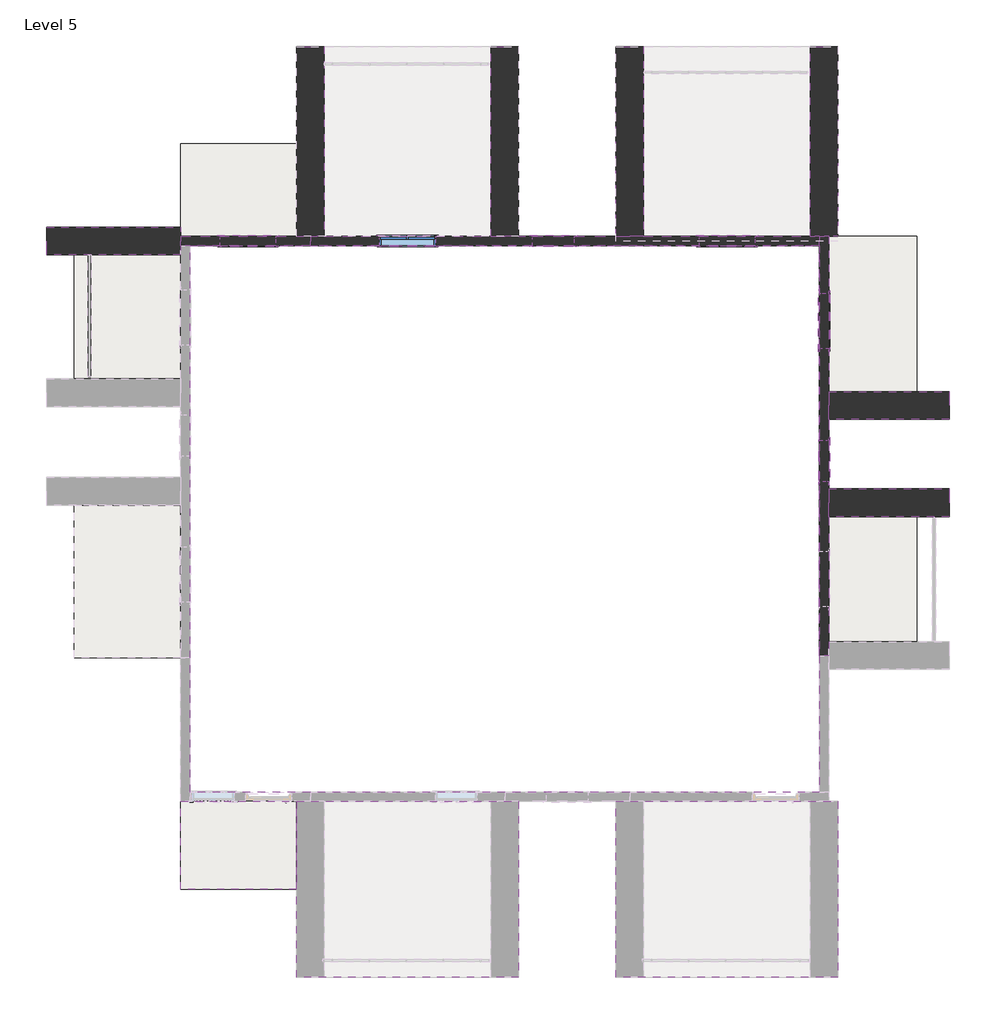
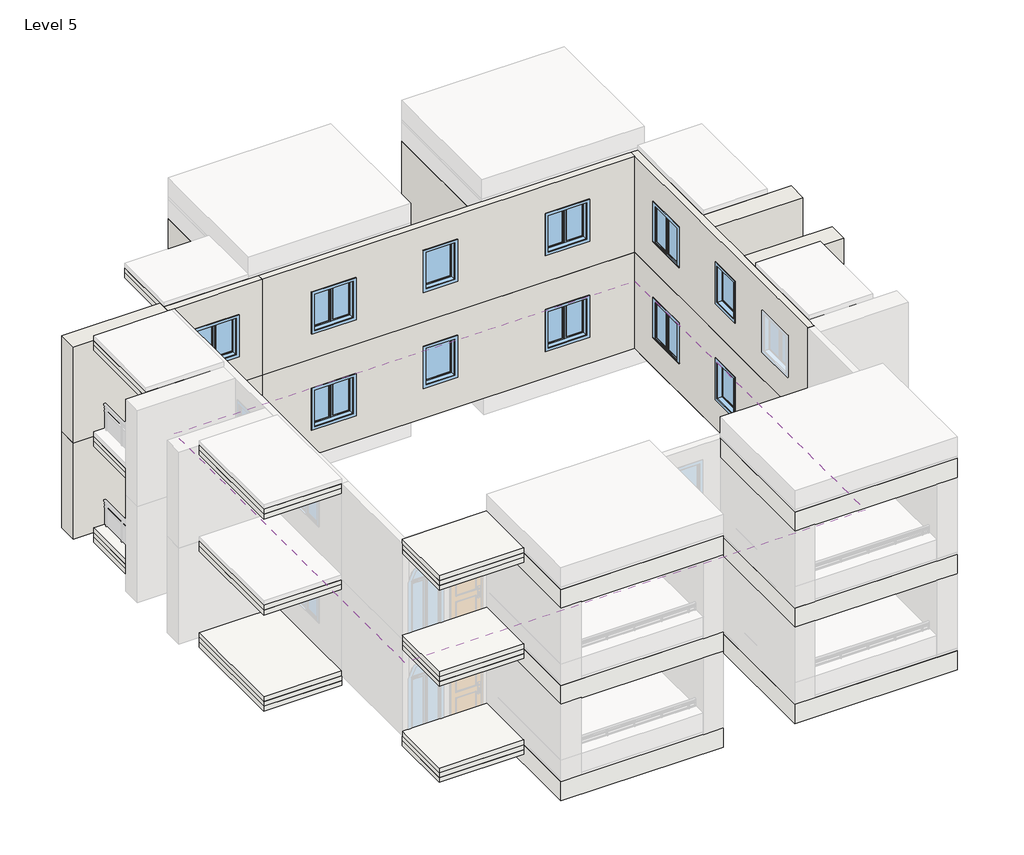
# One storey, part 2 of 4: 20 walls, 16 slabs, 12 windows, 1 covering.
"""IFC4 building model written with IfcOpenShell, lengths in millimetres."""

from ifc_helpers import new_model, si_unit, frame, origin, place, context, project, spatial, polyline, outline, extrude, faceted_brep, transform, mapped, element, save
from components import window_0862ab64, window_3a1167bf, window_8a4441b2

model = new_model("IFC4")

# Units and contexts
model_context = context("Model", 3, world=origin())
ifc_project = project(units=[si_unit("LENGTHUNIT", "METRE", prefix="MILLI")], contexts=[model_context])

# Site, building, storey
site = spatial("IfcSite", under=ifc_project)
building = spatial("IfcBuilding", under=site)
storey = spatial("IfcBuildingStorey", under=building, Name="Level 5", Elevation=12192.0)

# Covering
placement = place(None, origin())
element("IfcCovering", 1, ObjectType="2' x 4' ACT System", at=placement, inside=storey, context=model_context, shape_type="SweptSolid", body=[
    extrude(outline(polyline([(-12179.4937431, 6319.013611), (-9537.8937431, 6319.013611), (1638.1062569, 6319.013611), (1638.1062569, -2672.586389), (1638.1062569, -5669.786389), (-2527.4937431, -5669.786389), (-5270.6937431, -5669.786389), (-9537.8937431, -5669.786389), (-12179.4937431, -5669.786389), (-12179.4937431, -2723.386389), (-12179.4937431, 6319.013611)])), frame((0.0, 0.0, 14630.4), z_axis=(0.0, 0.0, 1.0), x_axis=(1.0, 0.0, 0.0)), (0.0, 0.0, 1.0), 57.15),
])

# Slabs
element("IfcSlab", 2, ObjectType="Generic - 2' 2", at=placement, inside=storey, context=model_context, shape_type="SweptSolid", body=[
    extrude(outline(polyline([(-4965.8937431, -9733.786389), (-9842.6937431, -9733.786389), (-9842.6937431, -5872.986389), (-4965.8937431, -5872.986389), (-4965.8937431, -9733.786389)])), frame((0.0, 0.0, 11887.2), z_axis=(0.0, 0.0, 1.0), x_axis=(1.0, 0.0, 0.0)), (0.0, 0.0, 1.0), 609.6),
])
element("IfcSlab", 3, ObjectType="Generic - 2' 2", at=placement, inside=storey, context=model_context, shape_type="SweptSolid", body=[
    extrude(outline(polyline([(2044.5062569, -9733.786389), (-2832.2937431, -9733.786389), (-2832.2937431, -5872.986389), (2044.5062569, -5872.986389), (2044.5062569, -9733.786389)])), frame((0.0, 0.0, 11887.2), z_axis=(0.0, 0.0, 1.0), x_axis=(1.0, 0.0, 0.0)), (0.0, 0.0, 1.0), 609.6),
])
element("IfcSlab", 4, ObjectType="Generic - 2' 2", at=placement, inside=storey, context=model_context, shape_type="SweptSolid", body=[
    extrude(outline(polyline([(-4965.8937431, -9733.786389), (-9842.6937431, -9733.786389), (-9842.6937431, -5872.986389), (-4965.8937431, -5872.986389), (-4965.8937431, -9733.786389)])), frame((0.0, 0.0, 14935.2), z_axis=(0.0, 0.0, 1.0), x_axis=(1.0, 0.0, 0.0)), (0.0, 0.0, 1.0), 609.6),
])
element("IfcSlab", 5, ObjectType="Generic - 2' 2", at=placement, inside=storey, context=model_context, shape_type="SweptSolid", body=[
    extrude(outline(polyline([(2044.5062569, -9733.786389), (-2832.2937431, -9733.786389), (-2832.2937431, -5872.986389), (2044.5062569, -5872.986389), (2044.5062569, -9733.786389)])), frame((0.0, 0.0, 14935.2), z_axis=(0.0, 0.0, 1.0), x_axis=(1.0, 0.0, 0.0)), (0.0, 0.0, 1.0), 609.6),
])
element("IfcSlab", 6, ObjectType="Generic - 2' 2", at=placement, inside=storey, context=model_context, shape_type="SweptSolid", body=[
    extrude(outline(polyline([(-4965.8937431, -9733.786389), (-9842.6937431, -9733.786389), (-9842.6937431, -5872.986389), (-4965.8937431, -5872.986389), (-4965.8937431, -9733.786389)])), frame((0.0, 0.0, 17983.2), z_axis=(0.0, 0.0, 1.0), x_axis=(1.0, 0.0, 0.0)), (0.0, 0.0, 1.0), 609.6),
])
element("IfcSlab", 7, ObjectType="Generic - 2' 2", at=placement, inside=storey, context=model_context, shape_type="SweptSolid", body=[
    extrude(outline(polyline([(2044.5062569, -9733.786389), (-2832.2937431, -9733.786389), (-2832.2937431, -5872.986389), (2044.5062569, -5872.986389), (2044.5062569, -9733.786389)])), frame((0.0, 0.0, 17983.2), z_axis=(0.0, 0.0, 1.0), x_axis=(1.0, 0.0, 0.0)), (0.0, 0.0, 1.0), 609.6),
])
element("IfcSlab", 8, ObjectType="general 6\"", at=placement, inside=storey, context=model_context, shape_type="SweptSolid", body=[
    extrude(outline(polyline([(-14722.8064179, 6115.813611), (-12382.6937431, 6115.813611), (-12382.6937431, 3398.013611), (-14722.8064179, 3398.013611), (-14722.8064179, 6115.813611)])), frame((0.0, 0.0, 12192.0), z_axis=(0.0, 0.0, 1.0), x_axis=(1.0, 0.0, 0.0)), (0.0, 0.0, 1.0), 152.4),
    extrude(outline(polyline([(-14722.8064179, 629.413611), (-12382.6937431, 629.413611), (-12382.6937431, -2723.386389), (-14722.8064179, -2723.386389), (-14722.8064179, 629.413611)])), frame((0.0, 0.0, 12192.0), z_axis=(0.0, 0.0, 1.0), x_axis=(1.0, 0.0, 0.0)), (0.0, 0.0, 1.0), 152.4),
    extrude(outline(polyline([(-9842.6937431, -5872.986389), (-9842.6937431, -7803.386389), (-12382.6937431, -7803.386389), (-12382.6937431, -5872.986389), (-9842.6937431, -5872.986389)])), frame((0.0, 0.0, 12192.0), z_axis=(0.0, 0.0, 1.0), x_axis=(1.0, 0.0, 0.0)), (0.0, 0.0, 1.0), 152.4),
    extrude(outline(polyline([(3771.7062569, -2367.786389), (1841.3062569, -2367.786389), (1841.3062569, 426.213611), (3771.7062569, 426.213611), (3771.7062569, -2367.786389)])), frame((0.0, 0.0, 12192.0), z_axis=(0.0, 0.0, 1.0), x_axis=(1.0, 0.0, 0.0)), (0.0, 0.0, 1.0), 152.4),
    extrude(outline(polyline([(3771.7062569, 3118.613611), (1841.3062569, 3118.613611), (1841.3062569, 6522.213611), (3771.7062569, 6522.213611), (3771.7062569, 3118.613611)])), frame((0.0, 0.0, 12192.0), z_axis=(0.0, 0.0, 1.0), x_axis=(1.0, 0.0, 0.0)), (0.0, 0.0, 1.0), 152.4),
    extrude(outline(polyline([(-12382.6937431, 6522.213611), (-12382.6937431, 8557.6995084), (-9842.6937431, 8557.6995084), (-9842.6937431, 6522.213611), (-12382.6937431, 6522.213611)])), frame((0.0, 0.0, 12192.0), z_axis=(0.0, 0.0, 1.0), x_axis=(1.0, 0.0, 0.0)), (0.0, 0.0, 1.0), 152.4),
])
element("IfcSlab", 9, ObjectType="general 6\"", at=placement, inside=storey, context=model_context, shape_type="SweptSolid", body=[
    extrude(outline(polyline([(-14722.8064179, 6115.813611), (-12382.6937431, 6115.813611), (-12382.6937431, 3398.013611), (-14722.8064179, 3398.013611), (-14722.8064179, 6115.813611)])), frame((0.0, 0.0, 15240.0), z_axis=(0.0, 0.0, 1.0), x_axis=(1.0, 0.0, 0.0)), (0.0, 0.0, 1.0), 152.4),
    extrude(outline(polyline([(-14722.8064179, 629.413611), (-12382.6937431, 629.413611), (-12382.6937431, -2723.386389), (-14722.8064179, -2723.386389), (-14722.8064179, 629.413611)])), frame((0.0, 0.0, 15240.0), z_axis=(0.0, 0.0, 1.0), x_axis=(1.0, 0.0, 0.0)), (0.0, 0.0, 1.0), 152.4),
    extrude(outline(polyline([(-9842.6937431, -5872.986389), (-9842.6937431, -7803.386389), (-12382.6937431, -7803.386389), (-12382.6937431, -5872.986389), (-9842.6937431, -5872.986389)])), frame((0.0, 0.0, 15240.0), z_axis=(0.0, 0.0, 1.0), x_axis=(1.0, 0.0, 0.0)), (0.0, 0.0, 1.0), 152.4),
    extrude(outline(polyline([(3771.7062569, -2367.786389), (1841.3062569, -2367.786389), (1841.3062569, 426.213611), (3771.7062569, 426.213611), (3771.7062569, -2367.786389)])), frame((0.0, 0.0, 15240.0), z_axis=(0.0, 0.0, 1.0), x_axis=(1.0, 0.0, 0.0)), (0.0, 0.0, 1.0), 152.4),
    extrude(outline(polyline([(3771.7062569, 3118.613611), (1841.3062569, 3118.613611), (1841.3062569, 6522.213611), (3771.7062569, 6522.213611), (3771.7062569, 3118.613611)])), frame((0.0, 0.0, 15240.0), z_axis=(0.0, 0.0, 1.0), x_axis=(1.0, 0.0, 0.0)), (0.0, 0.0, 1.0), 152.4),
    extrude(outline(polyline([(-12382.6937431, 6522.213611), (-12382.6937431, 8557.6995084), (-9842.6937431, 8557.6995084), (-9842.6937431, 6522.213611), (-12382.6937431, 6522.213611)])), frame((0.0, 0.0, 15240.0), z_axis=(0.0, 0.0, 1.0), x_axis=(1.0, 0.0, 0.0)), (0.0, 0.0, 1.0), 152.4),
])
element("IfcSlab", 10, ObjectType="general 6\"", at=placement, inside=storey, context=model_context, shape_type="SweptSolid", body=[
    extrude(outline(polyline([(-14722.8064179, 6115.813611), (-12382.6937431, 6115.813611), (-12382.6937431, 3398.013611), (-14722.8064179, 3398.013611), (-14722.8064179, 6115.813611)])), frame((0.0, 0.0, 18288.0), z_axis=(0.0, 0.0, 1.0), x_axis=(1.0, 0.0, 0.0)), (0.0, 0.0, 1.0), 152.4),
    extrude(outline(polyline([(-14722.8064179, 629.413611), (-12382.6937431, 629.413611), (-12382.6937431, -2723.386389), (-14722.8064179, -2723.386389), (-14722.8064179, 629.413611)])), frame((0.0, 0.0, 18288.0), z_axis=(0.0, 0.0, 1.0), x_axis=(1.0, 0.0, 0.0)), (0.0, 0.0, 1.0), 152.4),
    extrude(outline(polyline([(-9842.6937431, -5872.986389), (-9842.6937431, -7803.386389), (-12382.6937431, -7803.386389), (-12382.6937431, -5872.986389), (-9842.6937431, -5872.986389)])), frame((0.0, 0.0, 18288.0), z_axis=(0.0, 0.0, 1.0), x_axis=(1.0, 0.0, 0.0)), (0.0, 0.0, 1.0), 152.4),
    extrude(outline(polyline([(3771.7062569, -2367.786389), (1841.3062569, -2367.786389), (1841.3062569, 426.213611), (3771.7062569, 426.213611), (3771.7062569, -2367.786389)])), frame((0.0, 0.0, 18288.0), z_axis=(0.0, 0.0, 1.0), x_axis=(1.0, 0.0, 0.0)), (0.0, 0.0, 1.0), 152.4),
    extrude(outline(polyline([(3771.7062569, 3118.613611), (1841.3062569, 3118.613611), (1841.3062569, 6522.213611), (3771.7062569, 6522.213611), (3771.7062569, 3118.613611)])), frame((0.0, 0.0, 18288.0), z_axis=(0.0, 0.0, 1.0), x_axis=(1.0, 0.0, 0.0)), (0.0, 0.0, 1.0), 152.4),
    extrude(outline(polyline([(-12382.6937431, 6522.213611), (-12382.6937431, 8557.6995084), (-9842.6937431, 8557.6995084), (-9842.6937431, 6522.213611), (-12382.6937431, 6522.213611)])), frame((0.0, 0.0, 18288.0), z_axis=(0.0, 0.0, 1.0), x_axis=(1.0, 0.0, 0.0)), (0.0, 0.0, 1.0), 152.4),
])
element("IfcSlab", 11, ObjectType="general 6\" 2", at=placement, inside=storey, context=model_context, shape_type="SweptSolid", body=[
    extrude(outline(polyline([(3771.7062569, -2367.786389), (1841.3062569, -2367.786389), (1841.3062569, 375.413611), (3771.7062569, 375.413611), (3771.7062569, -2367.786389)])), frame((0.0, 0.0, 12344.4), z_axis=(0.0, 0.0, 1.0), x_axis=(1.0, 0.0, 0.0)), (0.0, 0.0, 1.0), 152.4),
    extrude(outline(polyline([(3771.7062569, 3118.613611), (1841.3062569, 3118.613611), (1841.3062569, 6522.213611), (3771.7062569, 6522.213611), (3771.7062569, 3118.613611)])), frame((0.0, 0.0, 12344.4), z_axis=(0.0, 0.0, 1.0), x_axis=(1.0, 0.0, 0.0)), (0.0, 0.0, 1.0), 152.4),
    extrude(outline(polyline([(-12382.6937431, 6522.213611), (-12382.6937431, 8557.6995084), (-9842.6937431, 8557.6995084), (-9842.6937431, 6522.213611), (-12382.6937431, 6522.213611)])), frame((0.0, 0.0, 12344.4), z_axis=(0.0, 0.0, 1.0), x_axis=(1.0, 0.0, 0.0)), (0.0, 0.0, 1.0), 152.4),
    extrude(outline(polyline([(-14722.8064179, 6115.813611), (-12384.3500805, 6115.813611), (-12384.3500805, 3398.013611), (-14722.8064179, 3398.013611), (-14722.8064179, 6115.813611)])), frame((0.0, 0.0, 12344.4), z_axis=(0.0, 0.0, 1.0), x_axis=(1.0, 0.0, 0.0)), (0.0, 0.0, 1.0), 152.4),
    extrude(outline(polyline([(-14722.8064179, -2723.386389), (-14722.8064179, 629.413611), (-12382.6937431, 629.413611), (-12382.6937431, -2723.386389), (-14722.8064179, -2723.386389)])), frame((0.0, 0.0, 12344.4), z_axis=(0.0, 0.0, 1.0), x_axis=(1.0, 0.0, 0.0)), (0.0, 0.0, 1.0), 152.4),
    extrude(outline(polyline([(-9842.6937431, -5872.986389), (-9842.6937431, -7803.386389), (-12382.6937431, -7803.386389), (-12382.6937431, -5872.986389), (-9842.6937431, -5872.986389)])), frame((0.0, 0.0, 12344.4), z_axis=(0.0, 0.0, 1.0), x_axis=(1.0, 0.0, 0.0)), (0.0, 0.0, 1.0), 152.4),
])
element("IfcSlab", 12, ObjectType="general 6\" 2", at=placement, inside=storey, context=model_context, shape_type="SweptSolid", body=[
    extrude(outline(polyline([(3771.7062569, -2367.786389), (1841.3062569, -2367.786389), (1841.3062569, 375.413611), (3771.7062569, 375.413611), (3771.7062569, -2367.786389)])), frame((0.0, 0.0, 15392.4), z_axis=(0.0, 0.0, 1.0), x_axis=(1.0, 0.0, 0.0)), (0.0, 0.0, 1.0), 152.4),
    extrude(outline(polyline([(3771.7062569, 3118.613611), (1841.3062569, 3118.613611), (1841.3062569, 6522.213611), (3771.7062569, 6522.213611), (3771.7062569, 3118.613611)])), frame((0.0, 0.0, 15392.4), z_axis=(0.0, 0.0, 1.0), x_axis=(1.0, 0.0, 0.0)), (0.0, 0.0, 1.0), 152.4),
    extrude(outline(polyline([(-12382.6937431, 6522.213611), (-12382.6937431, 8557.6995084), (-9842.6937431, 8557.6995084), (-9842.6937431, 6522.213611), (-12382.6937431, 6522.213611)])), frame((0.0, 0.0, 15392.4), z_axis=(0.0, 0.0, 1.0), x_axis=(1.0, 0.0, 0.0)), (0.0, 0.0, 1.0), 152.4),
    extrude(outline(polyline([(-14722.8064179, 6115.813611), (-12384.3500805, 6115.813611), (-12384.3500805, 3398.013611), (-14722.8064179, 3398.013611), (-14722.8064179, 6115.813611)])), frame((0.0, 0.0, 15392.4), z_axis=(0.0, 0.0, 1.0), x_axis=(1.0, 0.0, 0.0)), (0.0, 0.0, 1.0), 152.4),
    extrude(outline(polyline([(-14722.8064179, -2723.386389), (-14722.8064179, 629.413611), (-12382.6937431, 629.413611), (-12382.6937431, -2723.386389), (-14722.8064179, -2723.386389)])), frame((0.0, 0.0, 15392.4), z_axis=(0.0, 0.0, 1.0), x_axis=(1.0, 0.0, 0.0)), (0.0, 0.0, 1.0), 152.4),
    extrude(outline(polyline([(-9842.6937431, -5872.986389), (-9842.6937431, -7803.386389), (-12382.6937431, -7803.386389), (-12382.6937431, -5872.986389), (-9842.6937431, -5872.986389)])), frame((0.0, 0.0, 15392.4), z_axis=(0.0, 0.0, 1.0), x_axis=(1.0, 0.0, 0.0)), (0.0, 0.0, 1.0), 152.4),
])
element("IfcSlab", 13, ObjectType="general 6\" 2", at=placement, inside=storey, context=model_context, shape_type="SweptSolid", body=[
    extrude(outline(polyline([(3771.7062569, -2367.786389), (1841.3062569, -2367.786389), (1841.3062569, 375.413611), (3771.7062569, 375.413611), (3771.7062569, -2367.786389)])), frame((0.0, 0.0, 18440.4), z_axis=(0.0, 0.0, 1.0), x_axis=(1.0, 0.0, 0.0)), (0.0, 0.0, 1.0), 152.4),
    extrude(outline(polyline([(3771.7062569, 3118.613611), (1841.3062569, 3118.613611), (1841.3062569, 6522.213611), (3771.7062569, 6522.213611), (3771.7062569, 3118.613611)])), frame((0.0, 0.0, 18440.4), z_axis=(0.0, 0.0, 1.0), x_axis=(1.0, 0.0, 0.0)), (0.0, 0.0, 1.0), 152.4),
    extrude(outline(polyline([(-12382.6937431, 6522.213611), (-12382.6937431, 8557.6995084), (-9842.6937431, 8557.6995084), (-9842.6937431, 6522.213611), (-12382.6937431, 6522.213611)])), frame((0.0, 0.0, 18440.4), z_axis=(0.0, 0.0, 1.0), x_axis=(1.0, 0.0, 0.0)), (0.0, 0.0, 1.0), 152.4),
    extrude(outline(polyline([(-14722.8064179, 6115.813611), (-12384.3500805, 6115.813611), (-12384.3500805, 3398.013611), (-14722.8064179, 3398.013611), (-14722.8064179, 6115.813611)])), frame((0.0, 0.0, 18440.4), z_axis=(0.0, 0.0, 1.0), x_axis=(1.0, 0.0, 0.0)), (0.0, 0.0, 1.0), 152.4),
    extrude(outline(polyline([(-14722.8064179, -2723.386389), (-14722.8064179, 629.413611), (-12382.6937431, 629.413611), (-12382.6937431, -2723.386389), (-14722.8064179, -2723.386389)])), frame((0.0, 0.0, 18440.4), z_axis=(0.0, 0.0, 1.0), x_axis=(1.0, 0.0, 0.0)), (0.0, 0.0, 1.0), 152.4),
    extrude(outline(polyline([(-9842.6937431, -5872.986389), (-9842.6937431, -7803.386389), (-12382.6937431, -7803.386389), (-12382.6937431, -5872.986389), (-9842.6937431, -5872.986389)])), frame((0.0, 0.0, 18440.4), z_axis=(0.0, 0.0, 1.0), x_axis=(1.0, 0.0, 0.0)), (0.0, 0.0, 1.0), 152.4),
])
element("IfcSlab", 14, ObjectType="general 6\" 3", at=placement, inside=storey, context=model_context, shape_type="SweptSolid", body=[
    extrude(outline(polyline([(3771.7062569, 3118.613611), (1841.3062569, 3118.613611), (1841.3062569, 6522.213611), (3771.7062569, 6522.213611), (3771.7062569, 3118.613611)])), frame((0.0, 0.0, 12496.8), z_axis=(0.0, 0.0, 1.0), x_axis=(1.0, 0.0, 0.0)), (0.0, 0.0, 1.0), 152.4),
    extrude(outline(polyline([(3771.7062569, -2367.786389), (1841.3062569, -2367.786389), (1841.3062569, 375.413611), (3771.7062569, 375.413611), (3771.7062569, -2367.786389)])), frame((0.0, 0.0, 12496.8), z_axis=(0.0, 0.0, 1.0), x_axis=(1.0, 0.0, 0.0)), (0.0, 0.0, 1.0), 152.4),
    extrude(outline(polyline([(-12382.6937431, 6522.213611), (-12382.6937431, 8557.6995084), (-9842.6937431, 8557.6995084), (-9842.6937431, 6522.213611), (-12382.6937431, 6522.213611)])), frame((0.0, 0.0, 12496.8), z_axis=(0.0, 0.0, 1.0), x_axis=(1.0, 0.0, 0.0)), (0.0, 0.0, 1.0), 152.4),
    extrude(outline(polyline([(-14722.8064179, 3398.013611), (-14722.8064179, 6115.813611), (-12384.3500805, 6115.813611), (-12384.3500805, 3398.013611), (-14722.8064179, 3398.013611)])), frame((0.0, 0.0, 12496.8), z_axis=(0.0, 0.0, 1.0), x_axis=(1.0, 0.0, 0.0)), (0.0, 0.0, 1.0), 152.4),
    extrude(outline(polyline([(-14722.8064179, -2723.386389), (-14722.8064179, 629.413611), (-12382.6937431, 629.413611), (-12382.6937431, -2723.386389), (-14722.8064179, -2723.386389)])), frame((0.0, 0.0, 12496.8), z_axis=(0.0, 0.0, 1.0), x_axis=(1.0, 0.0, 0.0)), (0.0, 0.0, 1.0), 152.4),
])
element("IfcSlab", 15, ObjectType="general 6\" 3", at=placement, inside=storey, context=model_context, shape_type="SweptSolid", body=[
    extrude(outline(polyline([(-12382.6937431, -5872.986389), (-9842.6937431, -5872.986389), (-9842.6937431, -7803.386389), (-12382.6937431, -7803.386389), (-12382.6937431, -5872.986389)])), frame((0.0, 0.0, 12496.8), z_axis=(0.0, 0.0, 1.0), x_axis=(1.0, 0.0, 0.0)), (0.0, 0.0, 1.0), 152.4),
])
element("IfcSlab", 16, ObjectType="general 6\" 3", at=placement, inside=storey, context=model_context, shape_type="SweptSolid", body=[
    extrude(outline(polyline([(-12382.6937431, -5872.986389), (-9842.6937431, -5872.986389), (-9842.6937431, -7803.386389), (-12382.6937431, -7803.386389), (-12382.6937431, -5872.986389)])), frame((0.0, 0.0, 15544.8), z_axis=(0.0, 0.0, 1.0), x_axis=(1.0, 0.0, 0.0)), (0.0, 0.0, 1.0), 152.4),
])
element("IfcSlab", 17, ObjectType="general 6\" 3", at=placement, inside=storey, context=model_context, shape_type="SweptSolid", body=[
    extrude(outline(polyline([(-12382.6937431, -5872.986389), (-9842.6937431, -5872.986389), (-9842.6937431, -7803.386389), (-12382.6937431, -7803.386389), (-12382.6937431, -5872.986389)])), frame((0.0, 0.0, 18592.8), z_axis=(0.0, 0.0, 1.0), x_axis=(1.0, 0.0, 0.0)), (0.0, 0.0, 1.0), 152.4),
])

# Walls
element("IfcWall", 18, ObjectType="Generic - 8\"", at=placement, inside=storey, context=model_context, shape_type="Brep", body=[
    faceted_brep([(-12382.6937431, 6319.013611, 12496.8), (-12179.4937431, 6319.013611, 12496.8), (-9537.8937431, 6319.013611, 12496.8), (-9537.8937431, 6319.013611, 15544.8), (-12179.4937431, 6319.013611, 15544.8), (-12382.6937431, 6319.013611, 15544.8), (-10299.8937431, 6319.013611, 14630.4), (-10299.8937431, 6319.013611, 13411.2), (-11519.0937431, 6319.013611, 13411.2), (-11519.0937431, 6319.013611, 14630.4), (-12382.6937431, 6522.213611, 12496.8), (-12382.6937431, 6522.213611, 15544.8), (-9537.8937431, 6522.213611, 15544.8), (-9537.8937431, 6522.213611, 12496.8), (-9842.6937431, 6522.213611, 12496.8), (-10299.8937431, 6522.213611, 14630.4), (-11519.0937431, 6522.213611, 14630.4), (-11519.0937431, 6522.213611, 13411.2), (-10299.8937431, 6522.213611, 13411.2)], [[[0, 1, 2, 3, 4, 5], [6, 7, 8, 9]], [[10, 11, 12, 13, 14], [15, 16, 17, 18]], [[2, 1, 0, 10, 14, 13]], [[5, 4, 3, 12, 11]], [[0, 5, 11, 10]], [[7, 6, 15, 18]], [[8, 7, 18, 17]], [[9, 8, 17, 16]], [[6, 9, 16, 15]], [[2, 13, 12, 3]]]),
])
element("IfcWall", 19, ObjectType="Generic - 8\"", at=placement, inside=storey, context=model_context, shape_type="Brep", body=[
    faceted_brep([(1638.1062569, 6522.213611, 15544.8), (1638.1062569, 6522.213611, 12496.8), (1638.1062569, 6319.013611, 12496.8), (1638.1062569, -2672.586389, 12496.8), (1638.1062569, -2672.586389, 15544.8), (1638.1062569, 6319.013611, 15544.8), (1638.1062569, 1137.413611, 14701.6747769), (1638.1062569, 1137.413611, 13482.4747769), (1638.1062569, 2051.813611, 13482.4747769), (1638.1062569, 2051.813611, 14701.6747769), (1638.1062569, -1605.786389, 14641.5712595), (1638.1062569, -1605.786389, 13422.3712595), (1638.1062569, -386.586389, 13422.3712595), (1638.1062569, -386.586389, 14641.5712595), (1638.1062569, 4058.413611, 14641.5712595), (1638.1062569, 4058.413611, 13422.3712595), (1638.1062569, 5277.613611, 13422.3712595), (1638.1062569, 5277.613611, 14641.5712595), (1841.3062569, 6522.213611, 12496.8), (1841.3062569, 6522.213611, 15544.8), (1841.3062569, 3118.613611, 15544.8), (1841.3062569, 2509.013611, 15544.8), (1841.3062569, 985.013611, 15544.8), (1841.3062569, 375.413611, 15544.8), (1841.3062569, -2367.786389, 15544.8), (1841.3062569, -2672.586389, 15544.8), (1841.3062569, -2672.586389, 12496.8), (1841.3062569, -2367.786389, 12496.8), (1841.3062569, 375.413611, 12496.8), (1841.3062569, 985.013611, 12496.8), (1841.3062569, 2509.013611, 12496.8), (1841.3062569, 3118.613611, 12496.8), (1841.3062569, 1137.413611, 14701.6747769), (1841.3062569, 2051.813611, 14701.6747769), (1841.3062569, 2051.813611, 13482.4747769), (1841.3062569, 1137.413611, 13482.4747769), (1841.3062569, -1605.786389, 14641.5712595), (1841.3062569, -386.586389, 14641.5712595), (1841.3062569, -386.586389, 13422.3712595), (1841.3062569, -1605.786389, 13422.3712595), (1841.3062569, 4058.413611, 14641.5712595), (1841.3062569, 5277.613611, 14641.5712595), (1841.3062569, 5277.613611, 13422.3712595), (1841.3062569, 4058.413611, 13422.3712595)], [[[0, 1, 2, 3, 4, 5], [6, 7, 8, 9], [10, 11, 12, 13], [14, 15, 16, 17]], [[18, 19, 20, 21, 22, 23, 24, 25, 26, 27, 28, 29, 30, 31], [32, 33, 34, 35], [36, 37, 38, 39], [40, 41, 42, 43]], [[3, 2, 1, 18, 31, 30, 29, 28, 27, 26]], [[4, 3, 26, 25]], [[0, 5, 4, 25, 24, 23, 22, 21, 20, 19]], [[0, 19, 18, 1]], [[7, 6, 32, 35]], [[8, 7, 35, 34]], [[9, 8, 34, 33]], [[6, 9, 33, 32]], [[11, 10, 36, 39]], [[12, 11, 39, 38]], [[13, 12, 38, 37]], [[10, 13, 37, 36]], [[15, 14, 40, 43]], [[16, 15, 43, 42]], [[17, 16, 42, 41]], [[14, 17, 41, 40]]]),
])
element("IfcWall", 20, ObjectType="Generic - 8\"", at=placement, inside=storey, context=model_context, shape_type="Brep", body=[
    faceted_brep([(-9537.8937431, 6319.013611, 15544.8), (-9537.8937431, 6319.013611, 12496.8), (1638.1062569, 6319.013611, 12496.8), (1638.1062569, 6319.013611, 15544.8), (-3746.6937431, 6319.013611, 14728.3983257), (-3746.6937431, 6319.013611, 13509.1983257), (-4661.0937431, 6319.013611, 13509.1983257), (-4661.0937431, 6319.013611, 14728.3983257), (-6794.6937431, 6319.013611, 14577.182989), (-6794.6937431, 6319.013611, 13357.982989), (-8013.8937431, 6319.013611, 13357.982989), (-8013.8937431, 6319.013611, 14577.182989), (215.7062569, 6319.013611, 14614.4159819), (215.7062569, 6319.013611, 13395.2159819), (-1003.4937431, 6319.013611, 13395.2159819), (-1003.4937431, 6319.013611, 14614.4159819), (-9537.8937431, 6522.213611, 12496.8), (-9537.8937431, 6522.213611, 15544.8), (1638.1062569, 6522.213611, 15544.8), (1638.1062569, 6522.213611, 12496.8), (1434.9062569, 6522.213611, 12496.8), (-2222.6937431, 6522.213611, 12496.8), (-2832.2937431, 6522.213611, 12496.8), (-4965.8937431, 6522.213611, 12496.8), (-5575.4937431, 6522.213611, 12496.8), (-9233.0937431, 6522.213611, 12496.8), (-3746.6937431, 6522.213611, 14728.3983257), (-4661.0937431, 6522.213611, 14728.3983257), (-4661.0937431, 6522.213611, 13509.1983257), (-3746.6937431, 6522.213611, 13509.1983257), (-6794.6937431, 6522.213611, 14577.182989), (-8013.8937431, 6522.213611, 14577.182989), (-8013.8937431, 6522.213611, 13357.982989), (-6794.6937431, 6522.213611, 13357.982989), (215.7062569, 6522.213611, 14614.4159819), (-1003.4937431, 6522.213611, 14614.4159819), (-1003.4937431, 6522.213611, 13395.2159819), (215.7062569, 6522.213611, 13395.2159819)], [[[0, 1, 2, 3], [4, 5, 6, 7], [8, 9, 10, 11], [12, 13, 14, 15]], [[16, 17, 18, 19, 20, 21, 22, 23, 24, 25], [26, 27, 28, 29], [30, 31, 32, 33], [34, 35, 36, 37]], [[2, 1, 16, 25, 24, 23, 22, 21, 20, 19]], [[0, 3, 18, 17]], [[2, 19, 18, 3]], [[5, 4, 26, 29]], [[6, 5, 29, 28]], [[7, 6, 28, 27]], [[4, 7, 27, 26]], [[9, 8, 30, 33]], [[10, 9, 33, 32]], [[11, 10, 32, 31]], [[8, 11, 31, 30]], [[13, 12, 34, 37]], [[14, 13, 37, 36]], [[15, 14, 36, 35]], [[12, 15, 35, 34]], [[0, 17, 16, 1]]]),
])
element("IfcWall", 21, ObjectType="Generic - 8\"", at=placement, inside=storey, context=model_context, shape_type="Brep", body=[
    faceted_brep([(-12382.6937431, 6319.013611, 15544.8), (-12179.4937431, 6319.013611, 15544.8), (-9537.8937431, 6319.013611, 15544.8), (-9537.8937431, 6319.013611, 18592.8), (-12179.4937431, 6319.013611, 18592.8), (-12382.6937431, 6319.013611, 18592.8), (-10299.8937431, 6319.013611, 17678.4), (-10299.8937431, 6319.013611, 16459.2), (-11519.0937431, 6319.013611, 16459.2), (-11519.0937431, 6319.013611, 17678.4), (-12382.6937431, 6522.213611, 15544.8), (-12382.6937431, 6522.213611, 18592.8), (-9537.8937431, 6522.213611, 18592.8), (-9537.8937431, 6522.213611, 15544.8), (-9842.6937431, 6522.213611, 15544.8), (-10299.8937431, 6522.213611, 17678.4), (-11519.0937431, 6522.213611, 17678.4), (-11519.0937431, 6522.213611, 16459.2), (-10299.8937431, 6522.213611, 16459.2)], [[[0, 1, 2, 3, 4, 5], [6, 7, 8, 9]], [[10, 11, 12, 13, 14], [15, 16, 17, 18]], [[2, 1, 0, 10, 14, 13]], [[5, 4, 3, 12, 11]], [[0, 5, 11, 10]], [[7, 6, 15, 18]], [[8, 7, 18, 17]], [[9, 8, 17, 16]], [[6, 9, 16, 15]], [[2, 13, 12, 3]]]),
])
element("IfcWall", 22, ObjectType="Generic - 8\"", at=placement, inside=storey, context=model_context, shape_type="Brep", body=[
    faceted_brep([(1638.1062569, 6522.213611, 18592.8), (1638.1062569, 6522.213611, 15544.8), (1638.1062569, 6319.013611, 15544.8), (1638.1062569, -2672.586389, 15544.8), (1638.1062569, -2672.586389, 18592.8), (1638.1062569, 6319.013611, 18592.8), (1638.1062569, 1137.413611, 17749.6747769), (1638.1062569, 1137.413611, 16530.4747769), (1638.1062569, 2051.813611, 16530.4747769), (1638.1062569, 2051.813611, 17749.6747769), (1638.1062569, -1605.786389, 17689.5712595), (1638.1062569, -1605.786389, 16470.3712595), (1638.1062569, -386.586389, 16470.3712595), (1638.1062569, -386.586389, 17689.5712595), (1638.1062569, 4058.413611, 17689.5712595), (1638.1062569, 4058.413611, 16470.3712595), (1638.1062569, 5277.613611, 16470.3712595), (1638.1062569, 5277.613611, 17689.5712595), (1841.3062569, 6522.213611, 15544.8), (1841.3062569, 6522.213611, 18592.8), (1841.3062569, 3118.613611, 18592.8), (1841.3062569, 2509.013611, 18592.8), (1841.3062569, 985.013611, 18592.8), (1841.3062569, 375.413611, 18592.8), (1841.3062569, -2367.786389, 18592.8), (1841.3062569, -2672.586389, 18592.8), (1841.3062569, -2672.586389, 15544.8), (1841.3062569, -2367.786389, 15544.8), (1841.3062569, 375.413611, 15544.8), (1841.3062569, 985.013611, 15544.8), (1841.3062569, 2509.013611, 15544.8), (1841.3062569, 3118.613611, 15544.8), (1841.3062569, 1137.413611, 17749.6747769), (1841.3062569, 2051.813611, 17749.6747769), (1841.3062569, 2051.813611, 16530.4747769), (1841.3062569, 1137.413611, 16530.4747769), (1841.3062569, -1605.786389, 17689.5712595), (1841.3062569, -386.586389, 17689.5712595), (1841.3062569, -386.586389, 16470.3712595), (1841.3062569, -1605.786389, 16470.3712595), (1841.3062569, 4058.413611, 17689.5712595), (1841.3062569, 5277.613611, 17689.5712595), (1841.3062569, 5277.613611, 16470.3712595), (1841.3062569, 4058.413611, 16470.3712595)], [[[0, 1, 2, 3, 4, 5], [6, 7, 8, 9], [10, 11, 12, 13], [14, 15, 16, 17]], [[18, 19, 20, 21, 22, 23, 24, 25, 26, 27, 28, 29, 30, 31], [32, 33, 34, 35], [36, 37, 38, 39], [40, 41, 42, 43]], [[3, 2, 1, 18, 31, 30, 29, 28, 27, 26]], [[4, 3, 26, 25]], [[0, 5, 4, 25, 24, 23, 22, 21, 20, 19]], [[0, 19, 18, 1]], [[7, 6, 32, 35]], [[8, 7, 35, 34]], [[9, 8, 34, 33]], [[6, 9, 33, 32]], [[11, 10, 36, 39]], [[12, 11, 39, 38]], [[13, 12, 38, 37]], [[10, 13, 37, 36]], [[15, 14, 40, 43]], [[16, 15, 43, 42]], [[17, 16, 42, 41]], [[14, 17, 41, 40]]]),
])
element("IfcWall", 23, ObjectType="Generic - 8\"", at=placement, inside=storey, context=model_context, shape_type="Brep", body=[
    faceted_brep([(-9537.8937431, 6319.013611, 18592.8), (-9537.8937431, 6319.013611, 15544.8), (1638.1062569, 6319.013611, 15544.8), (1638.1062569, 6319.013611, 18592.8), (-3746.6937431, 6319.013611, 17776.3983257), (-3746.6937431, 6319.013611, 16557.1983257), (-4661.0937431, 6319.013611, 16557.1983257), (-4661.0937431, 6319.013611, 17776.3983257), (-6794.6937431, 6319.013611, 17625.182989), (-6794.6937431, 6319.013611, 16405.982989), (-8013.8937431, 6319.013611, 16405.982989), (-8013.8937431, 6319.013611, 17625.182989), (215.7062569, 6319.013611, 17662.4159819), (215.7062569, 6319.013611, 16443.2159819), (-1003.4937431, 6319.013611, 16443.2159819), (-1003.4937431, 6319.013611, 17662.4159819), (-9537.8937431, 6522.213611, 15544.8), (-9537.8937431, 6522.213611, 18592.8), (1638.1062569, 6522.213611, 18592.8), (1638.1062569, 6522.213611, 15544.8), (1434.9062569, 6522.213611, 15544.8), (-2222.6937431, 6522.213611, 15544.8), (-2832.2937431, 6522.213611, 15544.8), (-4965.8937431, 6522.213611, 15544.8), (-5575.4937431, 6522.213611, 15544.8), (-9233.0937431, 6522.213611, 15544.8), (-3746.6937431, 6522.213611, 17776.3983257), (-4661.0937431, 6522.213611, 17776.3983257), (-4661.0937431, 6522.213611, 16557.1983257), (-3746.6937431, 6522.213611, 16557.1983257), (-6794.6937431, 6522.213611, 17625.182989), (-8013.8937431, 6522.213611, 17625.182989), (-8013.8937431, 6522.213611, 16405.982989), (-6794.6937431, 6522.213611, 16405.982989), (215.7062569, 6522.213611, 17662.4159819), (-1003.4937431, 6522.213611, 17662.4159819), (-1003.4937431, 6522.213611, 16443.2159819), (215.7062569, 6522.213611, 16443.2159819)], [[[0, 1, 2, 3], [4, 5, 6, 7], [8, 9, 10, 11], [12, 13, 14, 15]], [[16, 17, 18, 19, 20, 21, 22, 23, 24, 25], [26, 27, 28, 29], [30, 31, 32, 33], [34, 35, 36, 37]], [[2, 1, 16, 25, 24, 23, 22, 21, 20, 19]], [[0, 3, 18, 17]], [[2, 19, 18, 3]], [[5, 4, 26, 29]], [[6, 5, 29, 28]], [[7, 6, 28, 27]], [[4, 7, 27, 26]], [[9, 8, 30, 33]], [[10, 9, 33, 32]], [[11, 10, 32, 31]], [[8, 11, 31, 30]], [[13, 12, 34, 37]], [[14, 13, 37, 36]], [[15, 14, 36, 35]], [[12, 15, 35, 34]], [[0, 17, 16, 1]]]),
])
element("IfcWall", 24, ObjectType="Generic -2' 2", at=placement, inside=storey, context=model_context, shape_type="Brep", body=[
    faceted_brep([(-12382.6937431, 6725.413611, 12496.8), (-15329.0937431, 6725.413611, 12496.8), (-15329.0937431, 6725.413611, 15544.8), (-12382.6937431, 6725.413611, 15544.8), (-12382.6937431, 6115.813611, 12496.8), (-12382.6937431, 6115.813611, 15544.8), (-15329.0937431, 6115.813611, 15544.8), (-15329.0937431, 6115.813611, 12496.8), (-12382.6937431, 6522.213611, 12496.8), (-12382.6937431, 6319.013611, 12496.8), (-12382.6937431, 6319.013611, 15544.8), (-12382.6937431, 6522.213611, 15544.8)], [[[0, 1, 2, 3]], [[4, 5, 6, 7]], [[1, 0, 8, 9, 4, 7]], [[2, 1, 7, 6]], [[3, 2, 6, 5, 10, 11]], [[0, 3, 11, 10, 5, 4, 9, 8]]]),
])
element("IfcWall", 25, ObjectType="Generic -2' 2", at=placement, inside=storey, context=model_context, shape_type="SweptSolid", body=[
    extrude(outline(polyline([(4482.9062569, 375.413611), (1841.3062569, 375.413611), (1841.3062569, 985.013611), (4482.9062569, 985.013611), (4482.9062569, 375.413611)])), frame((0.0, 0.0, 12496.8), z_axis=(0.0, 0.0, 1.0), x_axis=(1.0, 0.0, 0.0)), (0.0, 0.0, 1.0), 3048.0),
])
element("IfcWall", 26, ObjectType="Generic -2' 2", at=placement, inside=storey, context=model_context, shape_type="SweptSolid", body=[
    extrude(outline(polyline([(4482.9062569, 2509.013611), (1841.3062569, 2509.013611), (1841.3062569, 3118.613611), (4482.9062569, 3118.613611), (4482.9062569, 2509.013611)])), frame((0.0, 0.0, 12496.8), z_axis=(0.0, 0.0, 1.0), x_axis=(1.0, 0.0, 0.0)), (0.0, 0.0, 1.0), 3048.0),
])
element("IfcWall", 27, ObjectType="Generic -2' 2", at=placement, inside=storey, context=model_context, shape_type="Brep", body=[
    faceted_brep([(-12382.6937431, 6725.413611, 15544.8), (-15329.0937431, 6725.413611, 15544.8), (-15329.0937431, 6725.413611, 18592.8), (-12382.6937431, 6725.413611, 18592.8), (-12382.6937431, 6115.813611, 15544.8), (-12382.6937431, 6115.813611, 18592.8), (-15329.0937431, 6115.813611, 18592.8), (-15329.0937431, 6115.813611, 15544.8), (-12382.6937431, 6522.213611, 15544.8), (-12382.6937431, 6319.013611, 15544.8), (-12382.6937431, 6319.013611, 18592.8), (-12382.6937431, 6522.213611, 18592.8)], [[[0, 1, 2, 3]], [[4, 5, 6, 7]], [[1, 0, 8, 9, 4, 7]], [[2, 1, 7, 6]], [[3, 2, 6, 5, 10, 11]], [[0, 3, 11, 10, 5, 4, 9, 8]]]),
])
element("IfcWall", 28, ObjectType="Generic -2' 2", at=placement, inside=storey, context=model_context, shape_type="SweptSolid", body=[
    extrude(outline(polyline([(4482.9062569, 375.413611), (1841.3062569, 375.413611), (1841.3062569, 985.013611), (4482.9062569, 985.013611), (4482.9062569, 375.413611)])), frame((0.0, 0.0, 15544.8), z_axis=(0.0, 0.0, 1.0), x_axis=(1.0, 0.0, 0.0)), (0.0, 0.0, 1.0), 3048.0),
])
element("IfcWall", 29, ObjectType="Generic -2' 2", at=placement, inside=storey, context=model_context, shape_type="SweptSolid", body=[
    extrude(outline(polyline([(4482.9062569, 2509.013611), (1841.3062569, 2509.013611), (1841.3062569, 3118.613611), (4482.9062569, 3118.613611), (4482.9062569, 2509.013611)])), frame((0.0, 0.0, 15544.8), z_axis=(0.0, 0.0, 1.0), x_axis=(1.0, 0.0, 0.0)), (0.0, 0.0, 1.0), 3048.0),
])
element("IfcWall", 30, ObjectType="Generic -2' 3 red", at=placement, inside=storey, context=model_context, shape_type="Brep", body=[
    faceted_brep([(-9233.0937431, 6522.213611, 12496.8), (-9233.0937431, 10687.813611, 12496.8), (-9233.0937431, 10687.813611, 14935.2), (-9233.0937431, 6522.213611, 14935.2), (-9842.6937431, 6522.213611, 12496.8), (-9842.6937431, 6522.213611, 14935.2), (-9842.6937431, 10687.813611, 14935.2), (-9842.6937431, 10687.813611, 12496.8), (-9537.8937431, 6522.213611, 12496.8)], [[[0, 1, 2, 3]], [[4, 5, 6, 7]], [[1, 0, 8, 4, 7]], [[2, 1, 7, 6]], [[3, 2, 6, 5]], [[0, 3, 5, 4, 8]]]),
])
element("IfcWall", 31, ObjectType="Generic -2' 3 red", at=placement, inside=storey, context=model_context, shape_type="SweptSolid", body=[
    extrude(outline(polyline([(-4965.8937431, 10687.813611), (-4965.8937431, 6522.213611), (-5575.4937431, 6522.213611), (-5575.4937431, 10687.813611), (-4965.8937431, 10687.813611)])), frame((0.0, 0.0, 12496.8), z_axis=(0.0, 0.0, 1.0), x_axis=(1.0, 0.0, 0.0)), (0.0, 0.0, 1.0), 2443.0998934),
])
element("IfcWall", 32, ObjectType="Generic -2' 3 red", at=placement, inside=storey, context=model_context, shape_type="SweptSolid", body=[
    extrude(outline(polyline([(-2222.6937431, 10687.813611), (-2222.6937431, 6522.213611), (-2832.2937431, 6522.213611), (-2832.2937431, 10687.813611), (-2222.6937431, 10687.813611)])), frame((0.0, 0.0, 12496.8), z_axis=(0.0, 0.0, 1.0), x_axis=(1.0, 0.0, 0.0)), (0.0, 0.0, 1.0), 2443.7584708),
])
element("IfcWall", 33, ObjectType="Generic -2' 3 red", at=placement, inside=storey, context=model_context, shape_type="Brep", body=[
    faceted_brep([(2044.5062569, 6522.213611, 12496.8), (2044.5062569, 10687.813611, 12496.8), (2044.5062569, 10687.813611, 14935.2), (2044.5062569, 6522.213611, 14935.2), (1434.9062569, 6522.213611, 12496.8), (1434.9062569, 6522.213611, 14935.2), (1434.9062569, 10687.813611, 14935.2), (1434.9062569, 10687.813611, 12496.8), (1841.3062569, 6522.213611, 12496.8), (1638.1062569, 6522.213611, 12496.8)], [[[0, 1, 2, 3]], [[4, 5, 6, 7]], [[1, 0, 8, 9, 4, 7]], [[2, 1, 7, 6]], [[3, 2, 6, 5]], [[0, 3, 5, 4, 9, 8]]]),
])
element("IfcWall", 34, ObjectType="Generic -2' 3 red", at=placement, inside=storey, context=model_context, shape_type="Brep", body=[
    faceted_brep([(-9233.0937431, 6522.213611, 15544.8), (-9233.0937431, 10687.813611, 15544.8), (-9233.0937431, 10687.813611, 17983.2), (-9233.0937431, 6522.213611, 17983.2), (-9842.6937431, 6522.213611, 15544.8), (-9842.6937431, 6522.213611, 17983.2), (-9842.6937431, 10687.813611, 17983.2), (-9842.6937431, 10687.813611, 15544.8), (-9537.8937431, 6522.213611, 15544.8)], [[[0, 1, 2, 3]], [[4, 5, 6, 7]], [[1, 0, 8, 4, 7]], [[2, 1, 7, 6]], [[3, 2, 6, 5]], [[0, 3, 5, 4, 8]]]),
])
element("IfcWall", 35, ObjectType="Generic -2' 3 red", at=placement, inside=storey, context=model_context, shape_type="SweptSolid", body=[
    extrude(outline(polyline([(-4965.8937431, 10687.813611), (-4965.8937431, 6522.213611), (-5575.4937431, 6522.213611), (-5575.4937431, 10687.813611), (-4965.8937431, 10687.813611)])), frame((0.0, 0.0, 15544.8), z_axis=(0.0, 0.0, 1.0), x_axis=(1.0, 0.0, 0.0)), (0.0, 0.0, 1.0), 2443.0998934),
])
element("IfcWall", 36, ObjectType="Generic -2' 3 red", at=placement, inside=storey, context=model_context, shape_type="SweptSolid", body=[
    extrude(outline(polyline([(-2222.6937431, 10687.813611), (-2222.6937431, 6522.213611), (-2832.2937431, 6522.213611), (-2832.2937431, 10687.813611), (-2222.6937431, 10687.813611)])), frame((0.0, 0.0, 15544.8), z_axis=(0.0, 0.0, 1.0), x_axis=(1.0, 0.0, 0.0)), (0.0, 0.0, 1.0), 2443.7584708),
])
element("IfcWall", 37, ObjectType="Generic -2' 3 red", at=placement, inside=storey, context=model_context, shape_type="Brep", body=[
    faceted_brep([(2044.5062569, 6522.213611, 15544.8), (2044.5062569, 10687.813611, 15544.8), (2044.5062569, 10687.813611, 17983.2), (2044.5062569, 6522.213611, 17983.2), (1434.9062569, 6522.213611, 15544.8), (1434.9062569, 6522.213611, 17983.2), (1434.9062569, 10687.813611, 17983.2), (1434.9062569, 10687.813611, 15544.8), (1841.3062569, 6522.213611, 15544.8), (1638.1062569, 6522.213611, 15544.8)], [[[0, 1, 2, 3]], [[4, 5, 6, 7]], [[1, 0, 8, 9, 4, 7]], [[2, 1, 7, 6]], [[3, 2, 6, 5]], [[0, 3, 5, 4, 9, 8]]]),
])

# Windows
window_shape = window_0862ab64(model_context)
element("IfcWindow", 38, ObjectType="Casement Dbl with Trim.0001 : 48\" x 48\"", at=placement, inside=storey, context=model_context, shape_type="MappedRepresentation", body=[
    mapped(window_shape, transform((-7404.2937431, 6401.563611, 12443.582989), x_axis=(1.0, 0.0, 0.0), y_axis=(0.0, 1.0, 0.0), z_axis=(0.0, 0.0, 1.0))),
])
element("IfcWindow", 39, ObjectType="Casement Dbl with Trim.0001 : 48\" x 48\"", at=placement, inside=storey, context=model_context, shape_type="MappedRepresentation", body=[
    mapped(window_shape, transform((-393.8937431, 6401.563611, 12480.8159819), x_axis=(1.0, 0.0, 0.0), y_axis=(0.0, 1.0, 0.0), z_axis=(0.0, 0.0, 1.0))),
])
element("IfcWindow", 40, ObjectType="Casement Dbl with Trim.0001 : 48\" x 48\"", at=placement, inside=storey, context=model_context, shape_type="MappedRepresentation", body=[
    mapped(window_shape, transform((-10909.4937431, 6401.563611, 12496.8), x_axis=(1.0, 0.0, 0.0), y_axis=(0.0, 1.0, 0.0), z_axis=(0.0, 0.0, 1.0))),
])
element("IfcWindow", 41, ObjectType="Casement Dbl with Trim.0001 : 48\" x 48\"", at=placement, inside=storey, context=model_context, shape_type="MappedRepresentation", body=[
    mapped(window_shape, transform((-7404.2937431, 6401.563611, 15491.582989), x_axis=(1.0, 0.0, 0.0), y_axis=(0.0, 1.0, 0.0), z_axis=(0.0, 0.0, 1.0))),
])
element("IfcWindow", 42, ObjectType="Casement Dbl with Trim.0001 : 48\" x 48\"", at=placement, inside=storey, context=model_context, shape_type="MappedRepresentation", body=[
    mapped(window_shape, transform((-393.8937431, 6401.563611, 15528.8159819), x_axis=(1.0, 0.0, 0.0), y_axis=(0.0, 1.0, 0.0), z_axis=(0.0, 0.0, 1.0))),
])
element("IfcWindow", 43, ObjectType="Casement Dbl with Trim.0001 : 48\" x 48\"", at=placement, inside=storey, context=model_context, shape_type="MappedRepresentation", body=[
    mapped(window_shape, transform((-10909.4937431, 6401.563611, 15544.8), x_axis=(1.0, 0.0, 0.0), y_axis=(0.0, 1.0, 0.0), z_axis=(0.0, 0.0, 1.0))),
])
window_2_shape = window_3a1167bf(model_context)
element("IfcWindow", 44, ObjectType="Casement Dbl with Trim.0001 : 48\" x 48\"", at=placement, inside=storey, context=model_context, shape_type="MappedRepresentation", body=[
    mapped(window_2_shape, transform((1758.7562569, 4668.013611, 12507.9712595), x_axis=(0.0, -1.0, 0.0), y_axis=(1.0, 0.0, 0.0), z_axis=(0.0, 0.0, 1.0))),
])
element("IfcWindow", 45, ObjectType="Casement Dbl with Trim.0001 : 48\" x 48\"", at=placement, inside=storey, context=model_context, shape_type="MappedRepresentation", body=[
    mapped(window_2_shape, transform((1758.7562569, 4668.013611, 15555.9712595), x_axis=(0.0, -1.0, 0.0), y_axis=(1.0, 0.0, 0.0), z_axis=(0.0, 0.0, 1.0))),
])
window_3_shape = window_8a4441b2(model_context)
element("IfcWindow", 46, ObjectType="Casement with Trim : 36\" x 48\"", at=placement, inside=storey, context=model_context, shape_type="MappedRepresentation", body=[
    mapped(window_3_shape, transform((-4203.8937431, 6420.613611, 12594.7983257), x_axis=(1.0, 0.0, 0.0), y_axis=(0.0, 1.0, 0.0), z_axis=(0.0, 0.0, 1.0))),
])
element("IfcWindow", 47, ObjectType="Casement with Trim : 36\" x 48\"", at=placement, inside=storey, context=model_context, shape_type="MappedRepresentation", body=[
    mapped(window_3_shape, transform((1739.7062569, 1594.613611, 12568.0747769), x_axis=(0.0, -1.0, 0.0), y_axis=(1.0, 0.0, 0.0), z_axis=(0.0, 0.0, 1.0))),
])
element("IfcWindow", 48, ObjectType="Casement with Trim : 36\" x 48\"", at=placement, inside=storey, context=model_context, shape_type="MappedRepresentation", body=[
    mapped(window_3_shape, transform((-4203.8937431, 6420.613611, 15642.7983257), x_axis=(1.0, 0.0, 0.0), y_axis=(0.0, 1.0, 0.0), z_axis=(0.0, 0.0, 1.0))),
])
element("IfcWindow", 49, ObjectType="Casement with Trim : 36\" x 48\"", at=placement, inside=storey, context=model_context, shape_type="MappedRepresentation", body=[
    mapped(window_3_shape, transform((1739.7062569, 1594.613611, 15616.0747769), x_axis=(0.0, -1.0, 0.0), y_axis=(1.0, 0.0, 0.0), z_axis=(0.0, 0.0, 1.0))),
])

save(model, "model.ifc")

# Revit data of these elements
# Type "2' x 4' ACT System"
#   Assembly Code = "C3030210"
#   built-in parameter 1002203 = 1 (stored number, unit not read)
#   built-in parameter 1002202 = 1 (stored number, unit not read)
#   Layers, outside or top first: 0' - 1 5/8" "Default" (function 1); 0' - 0 5/8" "Acoustic Ceiling Tile 24 x 48" (function 5)
# Type "Generic - 2' 2"
#   Assembly Code = "B1010"
#   Function = 0
#   Layers, outside or top first: 2' - 0" "Damp-proofing" (function 1)
# Type "general 6\""
#   Assembly Code = "B1010"
#   Function = 0
#   Layers, outside or top first: 0' - 6" "Concrete Masonry Units" (function 1)
# Type "general 6\" 2"
#   Assembly Code = "B1010"
#   Function = 0
#   Layers, outside or top first: 0' - 6" "Damp-proofing" (function 1)
# Type "general 6\" 3"
#   Assembly Code = "B1010"
#   Function = 0
#   Layers, outside or top first: 0' - 6" "Door - Frame" (function 1)
# Type "Generic - 8\""
#   Assembly Code = "B2010"
#   Layers, outside or top first: 0' - 8" no material (function 1)
# Type "Generic -2' 2"
#   Assembly Code = "B2010"
#   Layers, outside or top first: 2' - 0" "Damp-proofing" (function 1)
# Type "Generic -2' 3 red"
#   Assembly Code = "B2010"
#   Layers, outside or top first: 2' - 0" "Damp-proofing" (function 1)
# Type "Casement Dbl with Trim.0001 : 48\" x 48\""
#   Type Mark = "23"
#   Construction Type Id = "GSP4R"
#   Assembly Code = "B2020100"
#   Analytic Construction = "1/8 in Pilkington single glazing"
#   Visual Light Transmittance = 0.9
#   Solar Heat Gain Coefficient = 0.78
#   Heat Transfer Coefficient (U) = 0.6496 BTU/(h·ft²·°F)
#   Height = 4' - 0"
#   Default Sill Height = 3' - 0"
#   Trim Projection - Ext. = 0' - 0 1/2"
#   Trim Projection - Int. = 0' - 0 3/4"
#   Trim Width - Exterior = 0' - 3 1/2"
#   Trim Width - Interior = 0' - 3 1/2"
#   Width = 4' - 0"
#   Window Inset = 0' - 0 3/4"
#   Define Thermal Properties by = 1
#   Glass Pane Material = Glass
#   Sash Material = Sash
#   Trim Exterior Material = Trim
#   Trim Interior Material = Trim
#   Wall Closure = (empty or 0)
# Type "Casement with Trim : 36\" x 48\""
#   Type Mark = "14"
#   Construction Type Id = "GSP4R"
#   Assembly Code = "B2020100"
#   Analytic Construction = "1/8 in Pilkington single glazing"
#   Visual Light Transmittance = 0.9
#   Solar Heat Gain Coefficient = 0.78
#   Heat Transfer Coefficient (U) = 0.6496 BTU/(h·ft²·°F)
#   Height = 4' - 0"
#   Default Sill Height = 3' - 0"
#   Trim Projection - Ext. = 0' - 0 1/2"
#   Trim Projection - Int. = 0' - 0 3/4"
#   Trim Width - Exterior = 0' - 3 1/2"
#   Trim Width - Interior = 0' - 3 1/2"
#   Width = 3' - 0"
#   Window Inset = 0' - 0 3/4"
#   Define Thermal Properties by = 1
#   Glass Pane Material = Glass
#   Sash Material = Sash
#   Trim Exterior Material = Trim
#   Trim Interior Material = Trim
#   Wall Closure = (empty or 0)
# Element 1 (IfcCovering, "2' x 4' ACT System")
#   Height Offset From Level = 8' - 0"
#   Phase Created = New Construction
#   Materials on its faces: "Acoustic Ceiling Tile 24 x 48", "Default"
# Elements 2, 3 (IfcSlab, "Generic - 2' 2")
#   Height Offset From Level = 1' - 0"
#   Phase Created = New Construction
#   Materials on its faces: "Gypsum Wall Board", "Damp-proofing"
# Elements 4, 5 (IfcSlab, "Generic - 2' 2")
#   Height Offset From Level = 11' - 0"
#   Phase Created = New Construction
#   Materials on its faces: "Gypsum Wall Board", "Damp-proofing"
# Elements 6, 7 (IfcSlab, "Generic - 2' 2")
#   Height Offset From Level = 21' - 0"
#   Phase Created = New Construction
#   Materials on its faces: "Gypsum Wall Board", "Damp-proofing"
# Element 8 (IfcSlab, "general 6\"")
#   built-in parameter 1001955 = 3.14159 (stored number, unit not read)
#   Height Offset From Level = 0' - 6"
#   Phase Created = New Construction
#   Materials on its faces: "Concrete Masonry Units"
# Element 9 (IfcSlab, "general 6\"")
#   built-in parameter 1001955 = 3.14159 (stored number, unit not read)
#   Height Offset From Level = 10' - 6"
#   Phase Created = New Construction
#   Materials on its faces: "Concrete Masonry Units"
# Element 10 (IfcSlab, "general 6\"")
#   built-in parameter 1001955 = 3.14159 (stored number, unit not read)
#   Height Offset From Level = 20' - 6"
#   Phase Created = New Construction
#   Materials on its faces: "Concrete Masonry Units"
# Element 11 (IfcSlab, "general 6\" 2")
#   Height Offset From Level = 1' - 0"
#   Phase Created = New Construction
#   Materials on its faces: "Damp-proofing"
# Element 12 (IfcSlab, "general 6\" 2")
#   Height Offset From Level = 11' - 0"
#   Phase Created = New Construction
#   Materials on its faces: "Damp-proofing"
# Element 13 (IfcSlab, "general 6\" 2")
#   Height Offset From Level = 21' - 0"
#   Phase Created = New Construction
#   Materials on its faces: "Damp-proofing"
# Element 14 (IfcSlab, "general 6\" 3")
#   Height Offset From Level = 1' - 6"
#   Phase Created = New Construction
#   Materials on its faces: "Door - Frame"
# Element 15 (IfcSlab, "general 6\" 3")
#   built-in parameter 1001955 = 3.14159 (stored number, unit not read)
#   Height Offset From Level = 1' - 6"
#   Phase Created = New Construction
#   Materials on its faces: "Door - Frame"
# Element 16 (IfcSlab, "general 6\" 3")
#   built-in parameter 1001955 = 3.14159 (stored number, unit not read)
#   Height Offset From Level = 11' - 6"
#   Phase Created = New Construction
#   Materials on its faces: "Door - Frame"
# Element 17 (IfcSlab, "general 6\" 3")
#   built-in parameter 1001955 = 3.14159 (stored number, unit not read)
#   Height Offset From Level = 21' - 6"
#   Phase Created = New Construction
#   Materials on its faces: "Door - Frame"
# Elements 18, 19, 20 (IfcWall, "Generic - 8\"")
#   built-in parameter 1001111 = 1' - 0"
#   Top Offset = 0' - 0"
#   Base Offset = 1' - 0"
#   Unconnected Height = 10' - 0"
#   wall height = 10' - 0"
#   Phase Created = New Construction
#   Base Constraint = Level 5
#   Materials on its faces: "Default Wall", "Tile, Porcelain, 4in", "Parking Stripe"
# Elements 21, 22, 23 (IfcWall, "Generic - 8\"")
#   built-in parameter 1001111 = 11' - 0"
#   Top Offset = 0' - 0"
#   Base Offset = 11' - 0"
#   Unconnected Height = 10' - 0"
#   wall height = 10' - 0"
#   Phase Created = New Construction
#   Base Constraint = Level 5
#   Materials on its faces: "Default Wall", "Tile, Porcelain, 4in", "Parking Stripe"
# Elements 24, 25, 26 (IfcWall, "Generic -2' 2")
#   built-in parameter 1001111 = 1' - 0"
#   Top Offset = 0' - 0"
#   Base Offset = 1' - 0"
#   Unconnected Height = 10' - 0"
#   wall height = 10' - 0"
#   Phase Created = New Construction
#   Base Constraint = Level 5
#   Materials on its faces: "Gypsum Wall Board", "Damp-proofing"
# Elements 27, 28, 29 (IfcWall, "Generic -2' 2")
#   built-in parameter 1001111 = 11' - 0"
#   Top Offset = 0' - 0"
#   Base Offset = 11' - 0"
#   Unconnected Height = 10' - 0"
#   wall height = 10' - 0"
#   Phase Created = New Construction
#   Base Constraint = Level 5
#   Materials on its faces: "Gypsum Wall Board", "Damp-proofing"
# Elements 30, 33 (IfcWall, "Generic -2' 3 red")
#   built-in parameter 1001111 = 1' - 0"
#   Top Offset = 0' - 0"
#   Base Offset = 1' - 0"
#   Unconnected Height = 8' - 0"
#   wall height = 8' - 0"
#   Phase Created = New Construction
#   Base Constraint = Level 5
#   Materials on its faces: "Damp-proofing"
# Element 31 (IfcWall, "Generic -2' 3 red")
#   built-in parameter 1001111 = 1' - 0"
#   Top Offset = 0' - 0"
#   Base Offset = 1' - 0"
#   Unconnected Height = 8' - 0.18504"
#   wall height = 8' - 0.18504"
#   Phase Created = New Construction
#   Base Constraint = Level 5
#   Materials on its faces: "Damp-proofing"
# Element 32 (IfcWall, "Generic -2' 3 red")
#   built-in parameter 1001111 = 1' - 0"
#   Top Offset = 0' - 0"
#   Base Offset = 1' - 0"
#   Unconnected Height = 8' - 0.21096"
#   wall height = 8' - 0.21096"
#   Phase Created = New Construction
#   Base Constraint = Level 5
#   Materials on its faces: "Damp-proofing"
# Elements 34, 37 (IfcWall, "Generic -2' 3 red")
#   built-in parameter 1001111 = 11' - 0"
#   Top Offset = 0' - 0"
#   Base Offset = 11' - 0"
#   Unconnected Height = 8' - 0"
#   wall height = 8' - 0"
#   Phase Created = New Construction
#   Base Constraint = Level 5
#   Materials on its faces: "Damp-proofing"
# Element 35 (IfcWall, "Generic -2' 3 red")
#   built-in parameter 1001111 = 11' - 0"
#   Top Offset = 0' - 0"
#   Base Offset = 11' - 0"
#   Unconnected Height = 8' - 0.18504"
#   wall height = 8' - 0.18504"
#   Phase Created = New Construction
#   Base Constraint = Level 5
#   Materials on its faces: "Damp-proofing"
# Element 36 (IfcWall, "Generic -2' 3 red")
#   built-in parameter 1001111 = 11' - 0"
#   Top Offset = 0' - 0"
#   Base Offset = 11' - 0"
#   Unconnected Height = 8' - 0.21096"
#   wall height = 8' - 0.21096"
#   Phase Created = New Construction
#   Base Constraint = Level 5
#   Materials on its faces: "Damp-proofing"
# Element 38 (IfcWindow, "Casement Dbl with Trim.0001 : 48\" x 48\"")
#   Mark = "51"
#   Phase Created = New Construction
#   Materials on its faces: "Sash", "Trim", "Glass"
# Element 39 (IfcWindow, "Casement Dbl with Trim.0001 : 48\" x 48\"")
#   Mark = "52"
#   Phase Created = New Construction
#   Materials on its faces: "Sash", "Trim", "Glass"
# Element 40 (IfcWindow, "Casement Dbl with Trim.0001 : 48\" x 48\"")
#   Mark = "55"
#   Phase Created = New Construction
#   Materials on its faces: "Sash", "Trim", "Glass"
# Element 41 (IfcWindow, "Casement Dbl with Trim.0001 : 48\" x 48\"")
#   Mark = "64"
#   Phase Created = New Construction
#   Materials on its faces: "Sash", "Trim", "Glass"
# Element 42 (IfcWindow, "Casement Dbl with Trim.0001 : 48\" x 48\"")
#   Mark = "65"
#   Phase Created = New Construction
#   Materials on its faces: "Sash", "Trim", "Glass"
# Element 43 (IfcWindow, "Casement Dbl with Trim.0001 : 48\" x 48\"")
#   Mark = "68"
#   Phase Created = New Construction
#   Materials on its faces: "Sash", "Trim", "Glass"
# Element 44 (IfcWindow, "Casement Dbl with Trim.0001 : 48\" x 48\"")
#   Mark = "54"
#   Phase Created = New Construction
#   Materials on its faces: "Sash", "Trim", "Glass"
# Element 45 (IfcWindow, "Casement Dbl with Trim.0001 : 48\" x 48\"")
#   Mark = "67"
#   Phase Created = New Construction
#   Materials on its faces: "Sash", "Trim", "Glass"
# Element 46 (IfcWindow, "Casement with Trim : 36\" x 48\"")
#   Mark = "47"
#   Phase Created = New Construction
#   Materials on its faces: "Sash", "Trim", "Glass"
# Element 47 (IfcWindow, "Casement with Trim : 36\" x 48\"")
#   Mark = "48"
#   Phase Created = New Construction
#   Materials on its faces: "Sash", "Trim", "Glass"
# Element 48 (IfcWindow, "Casement with Trim : 36\" x 48\"")
#   Mark = "60"
#   Phase Created = New Construction
#   Materials on its faces: "Sash", "Trim", "Glass"
# Element 49 (IfcWindow, "Casement with Trim : 36\" x 48\"")
#   Mark = "61"
#   Phase Created = New Construction
#   Materials on its faces: "Sash", "Trim", "Glass"
# Materials
#   "Default": colour RGB 127 127 127, transparency 0
#   "Acoustic Ceiling Tile 24 x 48": class "Generic", colour RGB 229 229 229, transparency 0, Description = "Acoustic Ceiling Tile 24 x 48", Cost = 0
